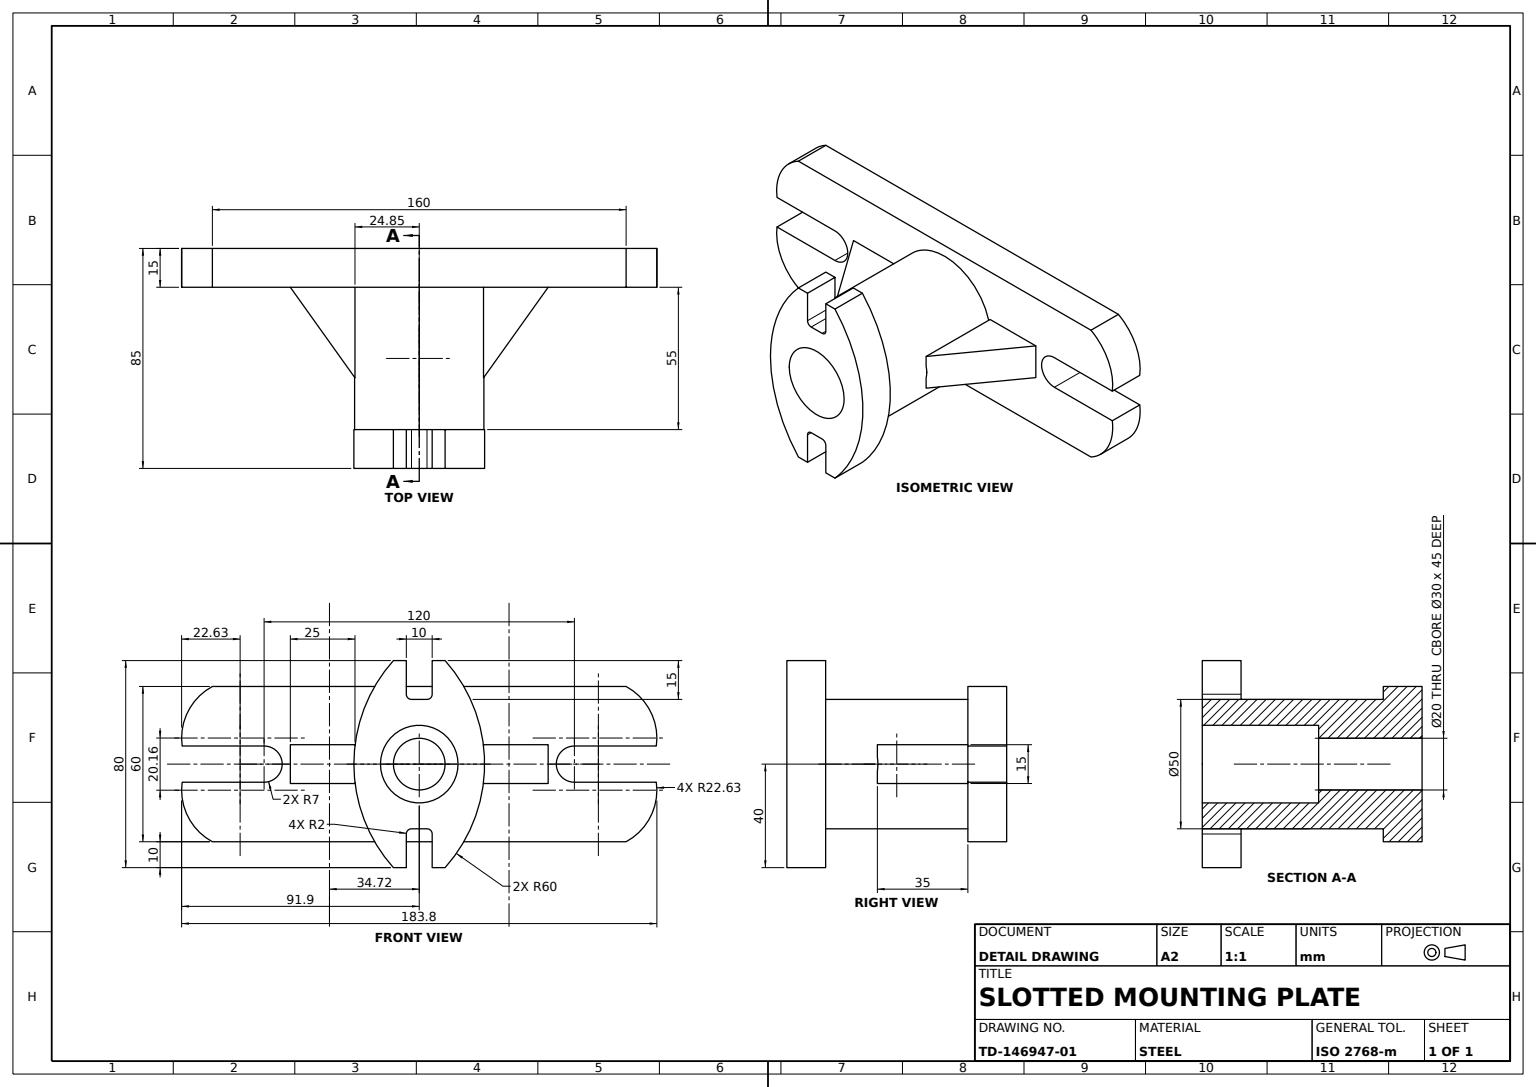
from build123d import *

# Parameters (mm, degrees)
FLANGE_PLATE_DEPTH            = 7.5
HUB_SKETCH_R                  = 25
HUB_50_DEPTH                  = 55
HUB_BORE_SKETCH_R             = 15
HUB_BORE_30_DEPTH             = 120.353625921
SLOTTED_START                 = 15
SLOTTED_COLLAR_SKETCH_R       = 15
SLOTTED_COLLAR_DEPTH          = 15
GUSSET_DEPTH                  = 7.5
COLLAR_FACE_BOSS_SKETCH_R     = 15
COLLAR_FACE_BOSS_DEPTH        = 85
THROUGH_BORE_20_SKETCH_R      = 10
THROUGH_BORE_20_DEPTH         = 132.416467844
COLLAR_BORE_30_SKETCH_R       = 15
COLLAR_BORE_30_DEPTH_45_DEPTH = 45


with BuildPart() as part:
    # Flange Plate Sketch → Flange Plate (new, symmetric)
    with BuildSketch(Plane.XY):
        with BuildLine():
            Line((-80, 30), (80, 30))
            ThreePointArc((80, 30), (89.443039653, 20.328945287), (91.687925992, 7))
            Line((91.687925992, 7), (60, 7))
            ThreePointArc((60, 7), (53, 0), (60, -7))
            Line((60, -7), (91.687925992, -7))
            ThreePointArc((91.687925992, -7), (89.443039653, -20.328945287), (80, -30))
            Line((80, -30), (-80, -30))
            ThreePointArc((-80, -30), (-89.443039653, -20.328945287), (-91.687925992, -7))
            Line((-91.687925992, -7), (-60, -7))
            ThreePointArc((-60, -7), (-53, 0), (-60, 7))
            Line((-60, 7), (-91.687925992, 7))
            ThreePointArc((-91.687925992, 7), (-89.443039653, 20.328945287), (-80, 30))
        make_face()
    extrude(amount=FLANGE_PLATE_DEPTH, both=True)

    # Hub Sketch → Hub Ø50 (add)
    with BuildSketch(Plane.XY.offset(7.5)):
        with Locations(Location((0, 0, 0), (0, 0, 180))):
            Circle(HUB_SKETCH_R)
    extrude(amount=HUB_50_DEPTH)

    # Hub Bore Sketch → Hub Bore Ø30 (cut, through all)
    with BuildSketch(Plane.XY.offset(62.5)):
        Circle(HUB_BORE_SKETCH_R)
    extrude(amount=-HUB_BORE_30_DEPTH, mode=Mode.SUBTRACT)

    # Slotted Collar Sketch → Slotted Collar (add)
    with BuildSketch(Plane.XY.offset(62.5).offset(SLOTTED_START)):
        with BuildLine():
            ThreePointArc((3, -25), (4.414213562, -25.585786438), (5, -27))
            Line((5, -27), (5, -40))
            Line((5, -40), (10, -40))
            ThreePointArc((10, -40), (25.27864045, 0), (10, 40))
            Line((10, 40), (5, 40))
            Line((5, 40), (5, 27))
            ThreePointArc((5, 27), (4.414213562, 25.585786438), (3, 25))
            Line((3, 25), (-3, 25))
            ThreePointArc((-3, 25), (-4.414213562, 25.585786438), (-5, 27))
            Line((-5, 27), (-5, 40))
            Line((-5, 40), (-10, 40))
            ThreePointArc((-10, 40), (-25.27864045, 0), (-10, -40))
            Line((-10, -40), (-5, -40))
            Line((-5, -40), (-5, -27))
            ThreePointArc((-5, -27), (-4.414213562, -25.585786438), (-3, -25))
            Line((-3, -25), (3, -25))
        make_face()
        Circle(SLOTTED_COLLAR_SKETCH_R, mode=Mode.SUBTRACT)
    extrude(amount=-SLOTTED_COLLAR_DEPTH)

    # Gusset Sketch → Gusset (add, symmetric)
    with BuildSketch(Plane(origin=(0, 0, 0), x_dir=(1, 0, 0), z_dir=(0, 1, 0))):
        Polygon((-24.85288252, -7.5), (-24.85288252, -42.5), (-49.85288252, -7.5), align=None)
    gusset = extrude(amount=GUSSET_DEPTH, both=True)

    # Gusset Mirror: Gusset across plane
    add(gusset.mirror(Plane(origin=(0, 0, 0), x_dir=(0, 0, 1), z_dir=(1, 0, 0))))

    # Collar Face Boss Sketch → Collar Face Boss (add, through all)
    with BuildSketch(Plane.XY.offset(77.5)):
        Circle(COLLAR_FACE_BOSS_SKETCH_R)
    extrude(amount=-COLLAR_FACE_BOSS_DEPTH)

    # Through Bore Ø20 Sketch → Through Bore Ø20 (cut, through all)
    with BuildSketch(Plane.XY.offset(77.5)):
        Circle(THROUGH_BORE_20_SKETCH_R)
    extrude(amount=-THROUGH_BORE_20_DEPTH, mode=Mode.SUBTRACT)

    # Collar Bore Ø30 Sketch → Collar Bore Ø30 Depth 45 (cut)
    with BuildSketch(Plane.XY.offset(77.5)):
        Circle(COLLAR_BORE_30_SKETCH_R)
    extrude(amount=-COLLAR_BORE_30_DEPTH_45_DEPTH, mode=Mode.SUBTRACT)


solid = part.part
